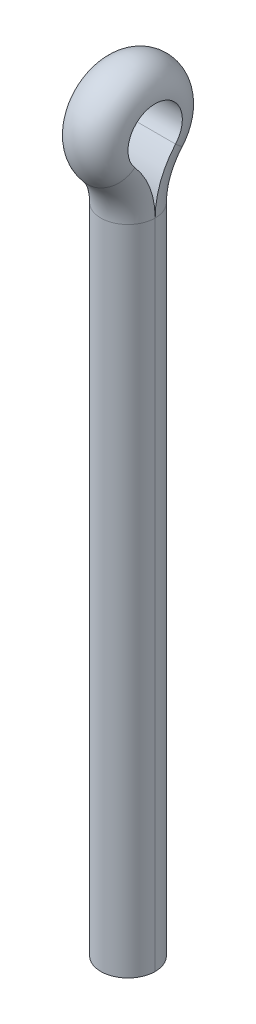
ISO-10303-21;
HEADER;
FILE_DESCRIPTION(('STEP AP214'),'2;1');
FILE_NAME('part.step','',(''),(''),'','','');
FILE_SCHEMA(('AUTOMOTIVE_DESIGN { 1 0 10303 214 1 1 1 1 }'));
ENDSEC;
DATA;
#1=APPLICATION_CONTEXT('core data for automotive mechanical design processes');
#2=APPLICATION_PROTOCOL_DEFINITION('international standard','automotive_design',2000,#1);
#3=PRODUCT_CONTEXT('',#1,'mechanical');
#4=PRODUCT('Part','Part','',(#3));
#5=PRODUCT_RELATED_PRODUCT_CATEGORY('part','',(#4));
#6=PRODUCT_DEFINITION_FORMATION('','',#4);
#7=PRODUCT_DEFINITION_CONTEXT('part definition',#1,'design');
#8=PRODUCT_DEFINITION('design','',#6,#7);
#9=PRODUCT_DEFINITION_SHAPE('','',#8);
#10=(LENGTH_UNIT() NAMED_UNIT(*) SI_UNIT(.MILLI.,.METRE.));
#11=(NAMED_UNIT(*) PLANE_ANGLE_UNIT() SI_UNIT($,.RADIAN.));
#12=(NAMED_UNIT(*) SI_UNIT($,.STERADIAN.) SOLID_ANGLE_UNIT());
#13=UNCERTAINTY_MEASURE_WITH_UNIT(LENGTH_MEASURE(1.E-05),#10,'distance_accuracy_value','');
#14=(GEOMETRIC_REPRESENTATION_CONTEXT(3) GLOBAL_UNCERTAINTY_ASSIGNED_CONTEXT((#13)) GLOBAL_UNIT_ASSIGNED_CONTEXT((#10,
#11,#12)) REPRESENTATION_CONTEXT('',''));
#15=CARTESIAN_POINT('',(0.,0.,0.));
#16=DIRECTION('',(0.,0.,1.));
#17=DIRECTION('',(1.,0.,0.));
#18=AXIS2_PLACEMENT_3D('',#15,#16,#17);
#19=CARTESIAN_POINT('',(0.,0.,0.));
#20=DIRECTION('',(0.,1.,0.));
#21=DIRECTION('',(0.,0.,1.));
#22=AXIS2_PLACEMENT_3D('',#19,#20,#21);
#23=PLANE('',#22);
#24=CARTESIAN_POINT('',(0.,0.,0.));
#25=DIRECTION('',(0.,1.,0.));
#26=DIRECTION('',(0.,0.,1.));
#27=AXIS2_PLACEMENT_3D('',#24,#25,#26);
#28=CIRCLE('',#27,1.5);
#29=CARTESIAN_POINT('',(1.5,0.,0.));
#30=VERTEX_POINT('',#29);
#31=CARTESIAN_POINT('',(-1.5,0.,0.));
#32=VERTEX_POINT('',#31);
#33=EDGE_CURVE('E60',#30,#32,#28,.T.);
#34=ORIENTED_EDGE('',*,*,#33,.F.);
#35=DIRECTION('',(1.,0.,0.));
#36=VECTOR('',#35,1.);
#37=CARTESIAN_POINT('',(-1.5,0.,0.));
#38=LINE('',#37,#36);
#39=EDGE_CURVE('E45',#32,#30,#38,.T.);
#40=ORIENTED_EDGE('',*,*,#39,.F.);
#41=EDGE_LOOP('',(#34,#40));
#42=FACE_BOUND('',#41,.T.);
#43=ADVANCED_FACE('F39',(#42),#23,.F.);
#44=CARTESIAN_POINT('',(0.,0.,0.));
#45=DIRECTION('',(0.,-1.,0.));
#46=DIRECTION('',(0.,0.,-1.));
#47=AXIS2_PLACEMENT_3D('',#44,#45,#46);
#48=PLANE('',#47);
#49=CARTESIAN_POINT('',(0.,0.,0.));
#50=DIRECTION('',(0.,-1.,0.));
#51=DIRECTION('',(0.,0.,-1.));
#52=AXIS2_PLACEMENT_3D('',#49,#50,#51);
#53=CIRCLE('',#52,1.5);
#54=EDGE_CURVE('E50',#30,#32,#53,.T.);
#55=ORIENTED_EDGE('',*,*,#54,.T.);
#56=ORIENTED_EDGE('',*,*,#39,.T.);
#57=EDGE_LOOP('',(#55,#56));
#58=FACE_BOUND('',#57,.T.);
#59=ADVANCED_FACE('F144',(#58),#48,.T.);
#60=CARTESIAN_POINT('',(0.,0.,0.));
#61=DIRECTION('',(0.,1.,0.));
#62=DIRECTION('',(0.,0.,1.));
#63=AXIS2_PLACEMENT_3D('',#60,#61,#62);
#64=CYLINDRICAL_SURFACE('',#63,1.5);
#65=DIRECTION('',(0.,-1.,0.));
#66=VECTOR('',#65,1.);
#67=CARTESIAN_POINT('',(-1.5,36.0313730334031,0.));
#68=LINE('',#67,#66);
#69=CARTESIAN_POINT('',(-1.5,36.0313730334031,0.));
#70=VERTEX_POINT('',#69);
#71=EDGE_CURVE('E11',#70,#32,#68,.T.);
#72=ORIENTED_EDGE('',*,*,#71,.F.);
#73=CARTESIAN_POINT('',(0.,36.0313730334031,0.));
#74=DIRECTION('',(0.,1.,0.));
#75=DIRECTION('',(0.,0.,1.));
#76=AXIS2_PLACEMENT_3D('',#73,#74,#75);
#77=CIRCLE('',#76,1.5);
#78=CARTESIAN_POINT('',(1.5,36.0313730334031,0.));
#79=VERTEX_POINT('',#78);
#80=EDGE_CURVE('E115',#79,#70,#77,.T.);
#81=ORIENTED_EDGE('',*,*,#80,.F.);
#82=DIRECTION('',(0.,-1.,0.));
#83=VECTOR('',#82,1.);
#84=CARTESIAN_POINT('',(1.5,36.0313730334031,0.));
#85=LINE('',#84,#83);
#86=EDGE_CURVE('E129',#79,#30,#85,.T.);
#87=ORIENTED_EDGE('',*,*,#86,.T.);
#88=ORIENTED_EDGE('',*,*,#33,.T.);
#89=EDGE_LOOP('',(#72,#81,#87,#88));
#90=FACE_BOUND('',#89,.T.);
#91=ADVANCED_FACE('F142',(#90),#64,.T.);
#92=CARTESIAN_POINT('',(0.,36.0313730334031,-4.5));
#93=DIRECTION('',(-1.,0.,0.));
#94=DIRECTION('',(0.,0.,1.));
#95=AXIS2_PLACEMENT_3D('',#92,#93,#94);
#96=TOROIDAL_SURFACE('',#95,4.5,1.5);
#97=CARTESIAN_POINT('',(-1.5,36.0313730334031,-4.5));
#98=DIRECTION('',(-1.,0.,0.));
#99=DIRECTION('',(0.,0.,1.));
#100=AXIS2_PLACEMENT_3D('',#97,#98,#99);
#101=CIRCLE('',#100,4.5);
#102=CARTESIAN_POINT('',(-1.5,39.0078432583508,-1.125));
#103=VERTEX_POINT('',#102);
#104=EDGE_CURVE('E98',#70,#103,#101,.T.);
#105=ORIENTED_EDGE('',*,*,#104,.T.);
#106=CARTESIAN_POINT('',(0.,39.0078432583508,-1.125));
#107=DIRECTION('',(0.,0.749999999999999,-0.661437827766148));
#108=DIRECTION('',(0.,0.661437827766148,0.749999999999999));
#109=AXIS2_PLACEMENT_3D('',#106,#107,#108);
#110=CIRCLE('',#109,1.5);
#111=CARTESIAN_POINT('',(1.5,39.0078432583508,-1.125));
#112=VERTEX_POINT('',#111);
#113=EDGE_CURVE('E82',#112,#103,#110,.T.);
#114=ORIENTED_EDGE('',*,*,#113,.F.);
#115=CARTESIAN_POINT('',(1.5,36.0313730334031,-4.5));
#116=DIRECTION('',(-1.,0.,0.));
#117=DIRECTION('',(0.,0.,1.));
#118=AXIS2_PLACEMENT_3D('',#115,#116,#117);
#119=CIRCLE('',#118,4.5);
#120=EDGE_CURVE('E102',#79,#112,#119,.T.);
#121=ORIENTED_EDGE('',*,*,#120,.F.);
#122=ORIENTED_EDGE('',*,*,#80,.T.);
#123=EDGE_LOOP('',(#105,#114,#121,#122));
#124=FACE_BOUND('',#123,.T.);
#125=ADVANCED_FACE('F105',(#124),#96,.T.);
#126=CARTESIAN_POINT('',(0.,36.0313730334031,-4.5));
#127=DIRECTION('',(-1.,0.,0.));
#128=DIRECTION('',(0.,0.,1.));
#129=AXIS2_PLACEMENT_3D('',#126,#127,#128);
#130=CYLINDRICAL_SURFACE('',#129,4.5);
#131=DIRECTION('',(1.,0.,0.));
#132=VECTOR('',#131,1.);
#133=CARTESIAN_POINT('',(-1.5,39.0078432583508,-1.125));
#134=LINE('',#133,#132);
#135=EDGE_CURVE('E90',#103,#112,#134,.T.);
#136=ORIENTED_EDGE('',*,*,#135,.F.);
#137=ORIENTED_EDGE('',*,*,#104,.F.);
#138=DIRECTION('',(1.,0.,0.));
#139=VECTOR('',#138,1.);
#140=CARTESIAN_POINT('',(-1.5,36.0313730334031,0.));
#141=LINE('',#140,#139);
#142=EDGE_CURVE('E109',#70,#79,#141,.T.);
#143=ORIENTED_EDGE('',*,*,#142,.T.);
#144=ORIENTED_EDGE('',*,*,#120,.T.);
#145=EDGE_LOOP('',(#136,#137,#143,#144));
#146=FACE_BOUND('',#145,.T.);
#147=ADVANCED_FACE('F107',(#146),#130,.T.);
#148=CARTESIAN_POINT('',(0.,40.,0.));
#149=DIRECTION('',(1.,0.,0.));
#150=DIRECTION('',(0.,0.,-1.));
#151=AXIS2_PLACEMENT_3D('',#148,#149,#150);
#152=TOROIDAL_SURFACE('',#151,1.50000000000001,1.5);
#153=CARTESIAN_POINT('',(-1.5,40.,0.));
#154=DIRECTION('',(1.,0.,0.));
#155=DIRECTION('',(0.,-0.66143782776615,-0.749999999999998));
#156=AXIS2_PLACEMENT_3D('',#153,#154,#155);
#157=CIRCLE('',#156,1.50000000000001);
#158=CARTESIAN_POINT('',(-1.5,39.0078432583508,1.12500000000001));
#159=VERTEX_POINT('',#158);
#160=EDGE_CURVE('E91',#103,#159,#157,.T.);
#161=ORIENTED_EDGE('',*,*,#160,.T.);
#162=CARTESIAN_POINT('',(0.,39.0078432583508,1.125));
#163=DIRECTION('',(0.,-0.75,-0.661437827766147));
#164=DIRECTION('',(0.,0.661437827766147,-0.75));
#165=AXIS2_PLACEMENT_3D('',#162,#163,#164);
#166=CIRCLE('',#165,1.5);
#167=CARTESIAN_POINT('',(1.5,39.0078432583508,1.12500000000001));
#168=VERTEX_POINT('',#167);
#169=EDGE_CURVE('E88',#168,#159,#166,.T.);
#170=ORIENTED_EDGE('',*,*,#169,.F.);
#171=CARTESIAN_POINT('',(1.5,40.,0.));
#172=DIRECTION('',(1.,0.,0.));
#173=DIRECTION('',(0.,-0.66143782776615,-0.749999999999998));
#174=AXIS2_PLACEMENT_3D('',#171,#172,#173);
#175=CIRCLE('',#174,1.50000000000001);
#176=EDGE_CURVE('E76',#112,#168,#175,.T.);
#177=ORIENTED_EDGE('',*,*,#176,.F.);
#178=ORIENTED_EDGE('',*,*,#113,.T.);
#179=EDGE_LOOP('',(#161,#170,#177,#178));
#180=FACE_BOUND('',#179,.T.);
#181=ADVANCED_FACE('F85',(#180),#152,.T.);
#182=CARTESIAN_POINT('',(0.,40.,0.));
#183=DIRECTION('',(1.,0.,0.));
#184=DIRECTION('',(0.,0.,-1.));
#185=AXIS2_PLACEMENT_3D('',#182,#183,#184);
#186=CYLINDRICAL_SURFACE('',#185,1.50000000000001);
#187=DIRECTION('',(1.,0.,0.));
#188=VECTOR('',#187,1.);
#189=CARTESIAN_POINT('',(-1.5,39.0078432583508,1.125));
#190=LINE('',#189,#188);
#191=EDGE_CURVE('E119',#159,#168,#190,.T.);
#192=ORIENTED_EDGE('',*,*,#191,.F.);
#193=ORIENTED_EDGE('',*,*,#160,.F.);
#194=ORIENTED_EDGE('',*,*,#135,.T.);
#195=ORIENTED_EDGE('',*,*,#176,.T.);
#196=EDGE_LOOP('',(#192,#193,#194,#195));
#197=FACE_BOUND('',#196,.T.);
#198=ADVANCED_FACE('F95',(#197),#186,.F.);
#199=CARTESIAN_POINT('',(0.,36.0313730334031,4.5));
#200=DIRECTION('',(-1.,0.,0.));
#201=DIRECTION('',(0.,0.,1.));
#202=AXIS2_PLACEMENT_3D('',#199,#200,#201);
#203=TOROIDAL_SURFACE('',#202,4.5,1.5);
#204=CARTESIAN_POINT('',(-1.5,36.0313730334031,4.5));
#205=DIRECTION('',(-1.,0.,0.));
#206=DIRECTION('',(0.,0.661437827766147,-0.750000000000001));
#207=AXIS2_PLACEMENT_3D('',#204,#205,#206);
#208=CIRCLE('',#207,4.5);
#209=EDGE_CURVE('E123',#159,#70,#208,.T.);
#210=ORIENTED_EDGE('',*,*,#209,.T.);
#211=CARTESIAN_POINT('',(0.,36.0313730334031,0.));
#212=DIRECTION('',(0.,-1.,0.));
#213=DIRECTION('',(0.,0.,-1.));
#214=AXIS2_PLACEMENT_3D('',#211,#212,#213);
#215=CIRCLE('',#214,1.5);
#216=EDGE_CURVE('E118',#79,#70,#215,.T.);
#217=ORIENTED_EDGE('',*,*,#216,.F.);
#218=CARTESIAN_POINT('',(1.5,36.0313730334031,4.5));
#219=DIRECTION('',(-1.,0.,0.));
#220=DIRECTION('',(0.,0.661437827766147,-0.750000000000001));
#221=AXIS2_PLACEMENT_3D('',#218,#219,#220);
#222=CIRCLE('',#221,4.5);
#223=EDGE_CURVE('E122',#168,#79,#222,.T.);
#224=ORIENTED_EDGE('',*,*,#223,.F.);
#225=ORIENTED_EDGE('',*,*,#169,.T.);
#226=EDGE_LOOP('',(#210,#217,#224,#225));
#227=FACE_BOUND('',#226,.T.);
#228=ADVANCED_FACE('F140',(#227),#203,.T.);
#229=CARTESIAN_POINT('',(0.,36.0313730334031,4.5));
#230=DIRECTION('',(-1.,0.,0.));
#231=DIRECTION('',(0.,0.,1.));
#232=AXIS2_PLACEMENT_3D('',#229,#230,#231);
#233=CYLINDRICAL_SURFACE('',#232,4.5);
#234=ORIENTED_EDGE('',*,*,#142,.F.);
#235=ORIENTED_EDGE('',*,*,#209,.F.);
#236=ORIENTED_EDGE('',*,*,#191,.T.);
#237=ORIENTED_EDGE('',*,*,#223,.T.);
#238=EDGE_LOOP('',(#234,#235,#236,#237));
#239=FACE_BOUND('',#238,.T.);
#240=ADVANCED_FACE('F133',(#239),#233,.T.);
#241=CARTESIAN_POINT('',(0.,36.0313730334031,0.));
#242=DIRECTION('',(0.,-1.,0.));
#243=DIRECTION('',(0.,0.,-1.));
#244=AXIS2_PLACEMENT_3D('',#241,#242,#243);
#245=CYLINDRICAL_SURFACE('',#244,1.5);
#246=ORIENTED_EDGE('',*,*,#71,.T.);
#247=ORIENTED_EDGE('',*,*,#54,.F.);
#248=ORIENTED_EDGE('',*,*,#86,.F.);
#249=ORIENTED_EDGE('',*,*,#216,.T.);
#250=EDGE_LOOP('',(#246,#247,#248,#249));
#251=FACE_BOUND('',#250,.T.);
#252=ADVANCED_FACE('F137',(#251),#245,.T.);
#253=CLOSED_SHELL('',(#43,#59,#91,#125,#147,#181,#198,#228,#240,#252));
#254=MANIFOLD_SOLID_BREP('B2',#253);
#255=ADVANCED_BREP_SHAPE_REPRESENTATION('',(#18,#254),#14);
#256=SHAPE_DEFINITION_REPRESENTATION(#9,#255);
ENDSEC;
END-ISO-10303-21;
